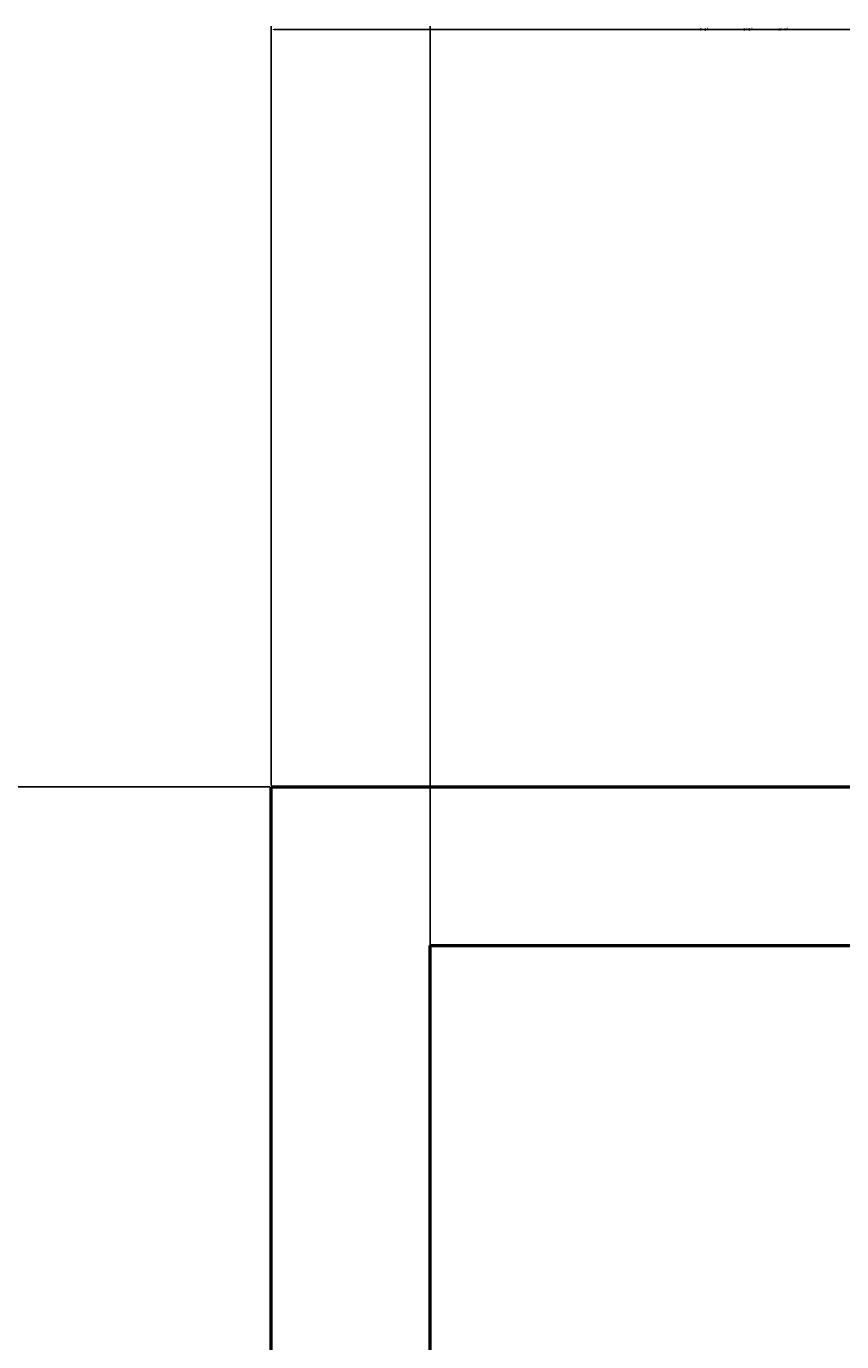
# Model space of a CAD drawing. Units: inches. Extents: x 37 to 824, y -700 to 234.
# Tile 56 of 77: x 147 to 193, y 160 to 234. Entities that reach past the tile are written whole.
import ezdxf

# ---------------------------------------------------------------- set-up
doc = ezdxf.new("R2010")
doc.units = ezdxf.units.IN
doc.header["$MEASUREMENT"] = 0
doc.layers.add('A-ANNO-DIMS', color=2, linetype='Continuous', lineweight=18)
doc.layers.add('A-WALL', color=2, linetype='Continuous', lineweight=50)
doc.styles.get("Standard").update_dxf_attribs({"font": 'arial.ttf'})
doc.dimstyles.get("Standard").update_dxf_attribs({"dimtxt": 0.18, "dimasz": 0.18, "dimexe": 0.18, "dimexo": 0.0625, "dimgap": 0.09, "dimtad": 0, "dimtih": 1, "dimtoh": 1, "dimdec": 1, "dimzin": 0, "dimdsep": 46, "dimlunit": 4, "dimtxsty": 'Standard', "dimcen": 0.09, "dimadec": 0, "dimazin": 0, "dimtfac": 1, "dimtdec": 1, "dimtofl": 0, "dimtmove": 0, "dimatfit": 3, "dimfxl": 1, "dimtolj": 1, "dimtzin": 0, "dimarcsym": 0})

# ---------------------------------------------------------------- blocks, each defined once
blk = doc.blocks.new('*D44')
at = {"layer": 'A-ANNO-DIMS', "color": 0, "lineweight": -2, "ltscale": 0.5, "transparency": 16777216}
for p, q in [((161.077, 191.153), (161.077, 234.17)), ((161.257, 233.99), (185.244, 233.99)), ((209.897, 233.99), (185.91, 233.99)), ((210.077, 191.153), (210.077, 234.17))]:
    blk.add_line(p, q, dxfattribs=at)
at = {"layer": 'A-ANNO-DIMS', "color": 0, "ltscale": 0.5, "transparency": 16777216}
for points in [[(161.257, 234.02), (161.257, 233.96), (161.077, 233.99)], [(209.897, 234.02), (209.897, 233.96), (210.077, 233.99)]]:
    blk.add_solid(points, dxfattribs=at)
at = {"layer": 'Defpoints', "color": 0, "ltscale": 0.5, "transparency": 16777216}
for p in [(210.077, 233.99), (161.077, 191.09), (210.077, 191.09)]:
    blk.add_point(p, dxfattribs=at)
at = {"layer": 'A-ANNO-DIMS', "color": 0, "ltscale": 0.5, "transparency": 16777216, "insert": (185.577, 233.99), "char_height": 0.18, "attachment_point": 5}
blk.add_mtext('\\A1;4\'-1"', dxfattribs=at)
blk = doc.blocks.new('*D49')
at = {"layer": 'A-ANNO-DIMS', "color": 0, "lineweight": -2, "ltscale": 0.5, "transparency": 16777216}
for p, q in [((161.015, 191.09), (78.159, 191.09)), ((78.339, 190.91), (78.339, 172.272)), ((78.339, 153.27), (78.339, 171.908)), ((161.015, 153.09), (78.159, 153.09))]:
    blk.add_line(p, q, dxfattribs=at)
at = {"layer": 'A-ANNO-DIMS', "color": 0, "ltscale": 0.5, "transparency": 16777216}
for points in [[(78.309, 190.91), (78.369, 190.91), (78.339, 191.09)], [(78.309, 153.27), (78.369, 153.27), (78.339, 153.09)]]:
    blk.add_solid(points, dxfattribs=at)
at = {"layer": 'Defpoints', "color": 0, "ltscale": 0.5, "transparency": 16777216}
for p in [(161.077, 191.09), (78.339, 153.09), (161.077, 153.09)]:
    blk.add_point(p, dxfattribs=at)
at = {"layer": 'A-ANNO-DIMS', "color": 0, "ltscale": 0.5, "transparency": 16777216, "insert": (78.339, 172.09), "char_height": 0.18, "attachment_point": 5}
blk.add_mtext('\\A1;3\'-2"', dxfattribs=at)
blk = doc.blocks.new('*D63')
at = {"layer": 'A-ANNO-DIMS', "color": 0, "lineweight": -2, "ltscale": 0.5, "transparency": 16777216}
for p, q in [((161.077, 191.153), (161.077, 234.17)), ((161.257, 233.99), (294.176, 233.99)), ((427.897, 233.99), (294.978, 233.99)), ((428.077, 191.153), (428.077, 234.17))]:
    blk.add_line(p, q, dxfattribs=at)
at = {"layer": 'A-ANNO-DIMS', "color": 0, "ltscale": 0.5, "transparency": 16777216}
for points in [[(161.257, 234.02), (161.257, 233.96), (161.077, 233.99)], [(427.897, 234.02), (427.897, 233.96), (428.077, 233.99)]]:
    blk.add_solid(points, dxfattribs=at)
at = {"layer": 'Defpoints', "color": 0, "ltscale": 0.5, "transparency": 16777216}
for p in [(428.077, 233.99), (161.077, 191.09), (428.077, 191.09)]:
    blk.add_point(p, dxfattribs=at)
at = {"layer": 'A-ANNO-DIMS', "color": 0, "ltscale": 0.5, "transparency": 16777216, "insert": (294.577, 233.99), "char_height": 0.18, "attachment_point": 5}
blk.add_mtext('\\A1;22\'-3"', dxfattribs=at)
blk = doc.blocks.new('*D72')
at = {"layer": 'A-ANNO-DIMS', "color": 0, "lineweight": -2, "ltscale": 0.5, "transparency": 16777216}
for p, q in [((170.077, 84.153), (170.077, 234.17)), ((170.257, 233.99), (209.804, 233.99)), ((250.01, 233.99), (210.463, 233.99)), ((250.19, 84.153), (250.19, 234.17))]:
    blk.add_line(p, q, dxfattribs=at)
at = {"layer": 'A-ANNO-DIMS', "color": 0, "ltscale": 0.5, "transparency": 16777216}
for points in [[(170.257, 234.02), (170.257, 233.96), (170.077, 233.99)], [(250.01, 234.02), (250.01, 233.96), (250.19, 233.99)]]:
    blk.add_solid(points, dxfattribs=at)
at = {"layer": 'Defpoints', "color": 0, "ltscale": 0.5, "transparency": 16777216}
for p in [(250.19, 233.99), (170.077, 84.09), (250.19, 84.09)]:
    blk.add_point(p, dxfattribs=at)
at = {"layer": 'A-ANNO-DIMS', "color": 0, "ltscale": 0.5, "transparency": 16777216, "insert": (210.133, 233.99), "char_height": 0.18, "attachment_point": 5}
blk.add_mtext('\\A1;6\'-8"', dxfattribs=at)
blk = doc.blocks.new('*D84')
at = {"layer": 'A-ANNO-DIMS', "color": 0, "lineweight": -2, "ltscale": 0.5, "transparency": 16777216}
for p, q in [((170.077, -265.847), (170.077, 234.17)), ((170.257, 233.99), (189.748, 233.99)), ((209.897, 233.99), (190.406, 233.99)), ((210.077, -265.847), (210.077, 234.17))]:
    blk.add_line(p, q, dxfattribs=at)
at = {"layer": 'A-ANNO-DIMS', "color": 0, "ltscale": 0.5, "transparency": 16777216}
for points in [[(170.257, 234.02), (170.257, 233.96), (170.077, 233.99)], [(209.897, 234.02), (209.897, 233.96), (210.077, 233.99)]]:
    blk.add_solid(points, dxfattribs=at)
at = {"layer": 'Defpoints', "color": 0, "ltscale": 0.5, "transparency": 16777216}
for p in [(210.077, 233.99), (170.077, -265.91), (210.077, -265.91)]:
    blk.add_point(p, dxfattribs=at)
at = {"layer": 'A-ANNO-DIMS', "color": 0, "ltscale": 0.5, "transparency": 16777216, "insert": (190.077, 233.99), "char_height": 0.18, "attachment_point": 5}
blk.add_mtext('\\A1;3\'-4"', dxfattribs=at)
blk = doc.blocks.new('*D85')
at = {"layer": 'A-ANNO-DIMS', "color": 0, "lineweight": -2, "ltscale": 0.5, "transparency": 16777216}
for p, q in [((170.077, -356.847), (170.077, 234.17)), ((170.257, 233.99), (187.748, 233.99)), ((205.897, 233.99), (188.406, 233.99)), ((206.077, -356.847), (206.077, 234.17))]:
    blk.add_line(p, q, dxfattribs=at)
at = {"layer": 'A-ANNO-DIMS', "color": 0, "ltscale": 0.5, "transparency": 16777216}
for points in [[(170.257, 234.02), (170.257, 233.96), (170.077, 233.99)], [(205.897, 234.02), (205.897, 233.96), (206.077, 233.99)]]:
    blk.add_solid(points, dxfattribs=at)
at = {"layer": 'Defpoints', "color": 0, "ltscale": 0.5, "transparency": 16777216}
for p in [(206.077, 233.99), (170.077, -356.91), (206.077, -356.91)]:
    blk.add_point(p, dxfattribs=at)
at = {"layer": 'A-ANNO-DIMS', "color": 0, "ltscale": 0.5, "transparency": 16777216, "insert": (188.077, 233.99), "char_height": 0.18, "attachment_point": 5}
blk.add_mtext('\\A1;3\'-0"', dxfattribs=at)

msp = doc.modelspace()

# ---------------------------------------------------------------- linework, layer by layer
at = {"layer": 'A-WALL'}
for p, q in [((161.077, 191.09), (299.077, 191.09)), ((161.077, 75.09), (161.077, 191.09)), ((170.077, 182.09), (290.077, 182.09)), ((170.077, 84.09), (170.077, 182.09))]:
    msp.add_line(p, q, dxfattribs=at)

# ---------------------------------------------------------------- dimensions: what is measured, and where the dimension line sits
at = {"layer": 'A-ANNO-DIMS', "ltscale": 0.5}
for base, p1, p2, picture, middle in [((210.077, 233.99), (161.077, 191.09), (210.077, 191.09), '*D44', (185.577, 233.99)), ((428.077, 233.99), (161.077, 191.09), (428.077, 191.09), '*D63', (294.577, 233.99)), ((250.19, 233.99), (170.077, 84.09), (250.19, 84.09), '*D72', (210.133, 233.99)), ((210.077, 233.99), (170.077, -265.91), (210.077, -265.91), '*D84', (190.077, 233.99)), ((206.077, 233.99), (170.077, -356.91), (206.077, -356.91), '*D85', (188.077, 233.99))]:
    dim = msp.add_linear_dim(base=base, p1=p1, p2=p2, dimstyle='Standard', override={"dimdec": 1, "dimlfac": 1, "dimrnd": 0, "dimzin": 1, "dimdsep": 46, "dimlunit": 4, "dimfrac": 2}, dxfattribs=at)
    dim.commit()
    dim.dimension.update_dxf_attribs({"geometry": picture, "text_midpoint": middle})
dim = msp.add_linear_dim(base=(78.339, 153.09), p1=(161.077, 191.09), p2=(161.077, 153.09), angle=90, dimstyle='Standard', override={"dimdec": 1, "dimlfac": 1, "dimrnd": 0, "dimzin": 1, "dimdsep": 46, "dimlunit": 4, "dimfrac": 2}, dxfattribs=at)
dim.commit()
dim.dimension.update_dxf_attribs({"geometry": '*D49', "text_midpoint": (78.339, 172.09)})

doc.saveas('drawing.dxf')
